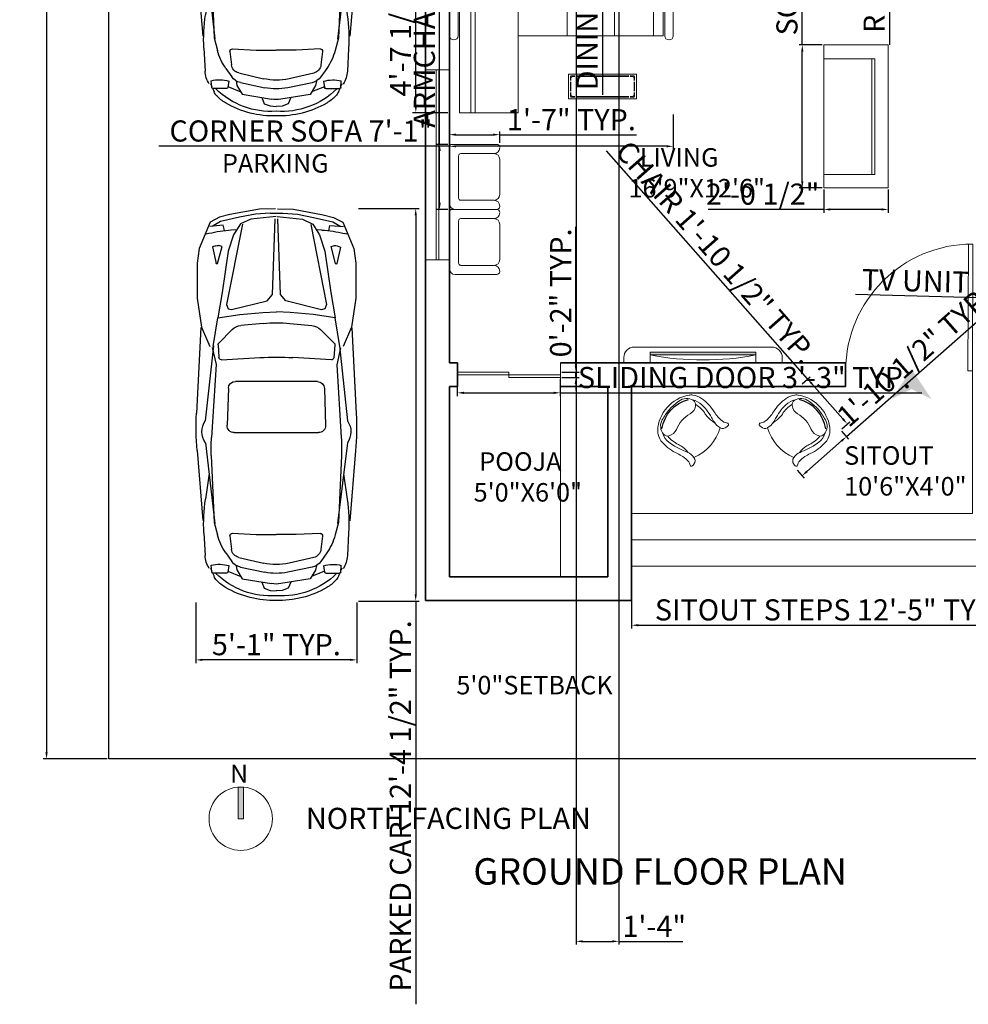
# Model space of a CAD drawing. Units: inches. Extents: x 3394 to 4794, y 965 to 1718.
# Tile 1 of 15: x 3394 to 3753, y 965 to 1338. Entities that reach past the tile are written whole.
import ezdxf

# ---------------------------------------------------------------- set-up
doc = ezdxf.new("R2010")
doc.units = ezdxf.units.IN
for name, color, linetype, lineweight in [('A-ANNO-DIMS', 2, 'Continuous', 13), ('A-ANNO-PATT', 1, 'Continuous', 13), ('A-ANNO-SYMB', 7, 'Continuous', 18), ('A-ANNO-TEXT', 7, 'Continuous', 18), ('A-ANNO-TITL', 7, 'Continuous', 25), ('A-AREA-IDEN', 7, 'Continuous', 18), ('A-DOOR', 4, 'Continuous', 18), ('A-EQPM', 8, 'Continuous', 18), ('A-EQPM-PATT', 8, 'Continuous', 13), ('A-FLOR-CASE', 8, 'Continuous', 18), ('A-FLOR-STRS', 7, 'Continuous', 18), ('A-GLAZ', 4, 'Continuous', 18), ('A-WALL', 7, 'Continuous', 35), ('C-PRKG-VEHI', 8, 'Continuous', 13), ('C-PROP', 7, 'Continuous', 25), ('NOITHAT', 21, 'Continuous', 18)]:
    doc.layers.add(name, color=color, linetype=linetype, lineweight=lineweight)
doc.layers.add('IFF-FURN-DETAIL', color=250, linetype='Continuous')
doc.layers.add('L9012X$0', color=2, linetype='Continuous')
doc.styles.get("Standard").update_dxf_attribs({"font": 'arial.ttf'})
doc.dimstyles.new('ISO-25', dxfattribs={"dimtxt": 8, "dimasz": 2.5, "dimexe": 1.25, "dimexo": 0.625, "dimtad": 1, "dimlunit": 3, "dimtxsty": 'Standard', "dimcen": 2.5, "dimadec": 0, "dimazin": 0, "dimtfac": 1, "dimtmove": 0, "dimatfit": 3, "dimfxl": 1, "dimarcsym": 0})

# ---------------------------------------------------------------- blocks, each defined once
blk = doc.blocks.new('sofa-27')
at = {"color": 0, "linetype": 'ByBlock'}
for p, q in [((0.094, 0.52), (0.459, 0.52)), ((-0.059, 0.059), (-0.059, 0.49)), ((0.035, 0.118), (0.035, 0.461)), ((0.518, 0.118), (0.518, 0.461)), ((0.613, 0.03), (0.613, 0.49)), ((0.583, 0), (0, 0)), ((0.494, 0.094), (0.059, 0.094))]:
    blk.add_line(p, q, dxfattribs=at)
for centre, radius, start, end in [((-0.03, 0.49), 0.0295, 90, 180), ((-0.024, 0.461), 0.0591, 360, 90), ((0.094, 0.461), 0.0591, 90, 180), ((0.459, 0.461), 0.0591, 0, 90), ((0.577, 0.461), 0.0591, 90, 180), ((0.583, 0.49), 0.0295, 0, 90), ((0.059, 0.118), 0.0236, 180, 270), ((0.494, 0.118), 0.0236, 270, 0), ((0, 0.059), 0.0591, 180, 270), ((0.583, 0.03), 0.0295, 270, 0)]:
    blk.add_arc(centre, radius, start, end, dxfattribs=at)
blk = doc.blocks.new('ILNG95')
for points in [[(120, 308, -0.32971), (51, 384, -0.036099), (50, 422, -0.497733), (75, 439, -0.070621), (96, 429, 0.101868), (133, 414, 0.091794), (259, 412, 0.024114), (351, 433, -0.090294), (638, 458, -0.132412), (775, 407, -0.068618), (816, 368, -0.184346), (943, 0, 1.803905)], [(120, 308, 0.138132), (244, 313, 0.001085), (325, 339, -0.034227), (462, 375, -0.033255), (567, 387, -0.137428), (727, 350, -4.561553)], [(120, 308, 0.138132), (244, 313, 0.001085), (325, 339, -0.034227), (462, 375, -0.033255), (567, 387, -0.137428), (727, 350, -4.561553)], [(235, 308, 0.064243), (394, 307, 0.04414), (433, 315, -0.118032), (643, 329, -6.296816)], [(235, 308, 0.064243), (394, 307, 0.04414), (433, 315, -0.118032), (643, 329, -6.296816)], [(639, 0, 0.078302), (612, 161, -0.233633), (633, 315, -0.28763), (710, 349, -0.317923), (875, 193, -0.032882), (900, 0, 1.140397)], [(639, 0, 0.078302), (612, 161, -0.233633), (633, 315, -0.28763), (710, 349, -0.317923), (875, 193, -0.032882), (900, 0, 1.140397)], [(120, -308, 0.32971), (51, -384, 0.036099), (50, -422, 0.497733), (75, -439, 0.070621), (96, -429, -0.101868), (133, -414, -0.091794), (259, -412, -0.024114), (351, -433, 0.090294), (638, -458, 0.132412), (775, -407, 0.068618), (816, -368, 0.184346), (943, 0, -1.803905)], [(639, 0, -0.078302), (612, -161, 0.233633), (633, -315, 0.28763), (710, -349, 0.317923), (875, -193, 0.032882), (900, 0, -1.140397)], [(639, 0, -0.078302), (612, -161, 0.233633), (633, -315, 0.28763), (710, -349, 0.317923), (875, -193, 0.032882), (900, 0, -1.140397)], [(120, -308, -0.138132), (244, -313, -0.001085), (325, -339, 0.034227), (462, -375, 0.033255), (567, -387, 0.137428), (727, -350, 4.561553)], [(120, -308, -0.138132), (244, -313, -0.001085), (325, -339, 0.034227), (462, -375, 0.033255), (567, -387, 0.137428), (727, -350, 4.561553)], [(235, -308, -0.064243), (394, -307, -0.04414), (433, -315, 0.118032), (643, -329, 6.296816)], [(235, -308, -0.064243), (394, -307, -0.04414), (433, -315, 0.118032), (643, -329, 6.296816)]]:
    blk.add_lwpolyline(points, format="xyb")
blk.add_arc((759, 1), 709, 154.3281, 205.801)
at = {"layer": 'IFF-FURN-DETAIL'}
blk.add_arc((326, -2), 549, 326.8997, 34.6691, dxfattribs=at)
blk.add_arc((326, -2), 549, 326.8997, 34.6691, dxfattribs=at)
blk = doc.blocks.new('A1099DC')
at = {"color": 0, "linetype": 'ByBlock'}
for p, q in [((1279.298465, 804.448389), (2201.430588, 851.890505)), ((272.228253, 749.073842), (265.114727, 718.465169)), ((1475.52921, 670.226262), (2282.402739, 758.004075)), ((2519.280414, 756.817792), (3387.476361, 653.818028)), ((2602.736326, 846.078152), (3356.693814, 785.353187)), ((2851.341839, 715.213377), (3126.60716, 755.701993)), ((3488.458929, 772.663345), (3732.658862, 759.86454)), ((139.051458, 595.027331), (190.951238, 683.213377)), ((179.200345, 564.515703), (190.951238, 709.631982)), ((398.733388, 644.315148), (411.280494, 678.748261)), ((411.280494, 678.748261), (588.616917, 641.417897)), ((1482.852352, 674.283145), (1175.286956, 622.180789)), ((1494.603245, 682.841284), (1678.210958, 641.166865)), ((1678.210958, 641.166865), (2462.684993, 690.847736)), ((2656.476214, 692.831247), (3376.704709, 662.004075)), ((3376.704709, 662.004075), (3510.708679, 626.736433)), ((3909.27561, 688.812956), (3837.725727, 693.401722)), ((3867.794139, 700.329656), (3900.059395, 686.767505)), ((3921.162781, 527.618662), (3921.162781, 676.138994)), ((3925.383812, 676.122818), (3955.306409, 663.545364)), ((92.537504, 388.14361), (139.051458, 595.027331)), ((236.043912, 551.980927), (179.200345, 564.515703)), ((405.405047, 577.538958), (396.874865, 615.894428)), ((589.014326, 626.599587), (405.405047, 577.538958)), ((1300.814287, 466.658131), (1445.712032, 613.104998)), ((1465.665584, 620.56924), (1602.893878, 610.287296)), ((1626.354615, 583.507504), (1602.652901, 169.222264)), ((3704.596898, 536.993674), (3795.675135, 473.385795)), ((229.117398, 477.634662), (225.714299, 427.957563)), ((1860.238743, -448.635916), (1859.369151, 433.397797)), ((1933.148906, 509.557888), (2330.980062, 522.200075)), ((2409.60024, 445.938054), (2410.49349, -460.09121)), ((3493.960271, 465.734554), (3507.923021, 209.166865)), ((3522.252709, 492.345257), (3666.066199, 475.644444)), ((3839.396146, 426.841284), (3888.358202, 417.538958)), ((3841.786866, 503.451367), (3910.58243, 515.096797)), ((3901.001848, 514.780764), (3957.150905, 375.772812)), ((57.774444, 216.608726), (92.537504, 388.14361)), ((1235.045743, 136.116317), (1257.419842, 373.755108)), ((3753.293176, 397.789551), (3815.226005, 132.124765)), ((3857.610793, 379.525702), (3912.067615, 118.157673)), ((3888.358202, 417.538958), (3983.199613, 359.957848)), ((3983.199613, 359.957848), (4035.448301, 43.94997)), ((49.168662, 58.00681), (57.774444, 216.608726)), ((3507.923021, 209.166865), (3507.64153, -4.333678)), ((4019.086894, 150.376168), (4084.69605, 122.469191)), ((4084.69605, 122.469191), (4109.177079, 60.329656)), ((4109.177079, 60.329656), (4113.094043, -5.158716)), ((49.301278, -76.507426), (58.219773, -235.092064)), ((3508.347273, -221.154823), (3507.644805, -7.65525)), ((3983.920268, -371.008369), (4035.545755, -54.898082)), ((4084.948231, -133.320044), (4109.306686, -71.132359)), ((4109.306686, -71.132359), (4113.094514, -5.636391)), ((1235.330373, -152.586046), (1258.173002, -390.180259)), ((1627.520644, -599.204785), (1603.002095, -184.967086)), ((3754.088875, -409.293325), (3815.497749, -143.506937)), ((3858.370276, -390.823819), (3912.311631, -129.348921)), ((4019.394229, -161.356334), (4084.948231, -133.320044)), ((58.219773, -235.092064), (93.320996, -406.558069)), ((3494.890446, -477.749545), (3508.347273, -221.154823)), ((93.320996, -406.558069), (140.24279, -613.349673)), ((3889.19258, -428.776374), (3983.920268, -371.008369)), ((3902.027941, -525.993061), (3957.902795, -386.874665)), ((230.077082, -495.779641), (226.576036, -446.109349)), ((1301.750547, -482.997536), (1446.936772, -629.158411)), ((1934.168526, -524.650381), (2332.023837, -536.508105)), ((3523.2353, -504.304409), (3667.01558, -487.320059)), ((3705.667171, -548.593196), (3796.61981, -484.805853)), ((3840.248961, -438.175225), (3889.19258, -428.776374)), ((3842.790735, -514.780444), (3911.609128, -526.290202)), ((140.24279, -613.349673), (192.316354, -701.433212)), ((237.150178, -570.112104), (180.331436, -582.758939)), ((180.331436, -582.758939), (192.368445, -727.851766)), ((406.561378, -595.336142), (398.106841, -633.708356)), ((590.267037, -644.034637), (406.561378, -595.336142)), ((1466.905004, -636.583294), (1604.112757, -626.030785)), ((3922.214148, -538.79118), (3922.506998, -687.311224)), ((273.723073, -767.133288), (266.549207, -736.538701)), ((400.0214, -662.125356), (412.636377, -696.533662)), ((412.636377, -696.533662), (589.898847, -658.853701)), ((1484.19765, -690.263206), (1176.530118, -638.767405)), ((1476.866524, -686.22077), (2283.911563, -772.40743)), ((1495.965396, -698.798158), (1679.490579, -656.761786)), ((1679.490579, -656.761786), (2464.061049, -704.895745)), ((2520.786439, -770.754078), (3388.777604, -666.042617)), ((2657.855804, -706.497136), (3378.022114, -674.249887)), ((2852.765183, -728.494989), (3128.109803, -768.440762)), ((3378.022114, -674.249887), (3511.956283, -638.718087)), ((3910.644841, -700.0086), (3839.104145, -704.738438)), ((3869.186159, -711.60707), (3901.424611, -697.981326)), ((3926.727989, -687.286725), (3956.625729, -674.650294)), ((1280.900818, -820.829563), (2203.124693, -866.453338)), ((2604.418191, -859.849707), (3358.254477, -797.638217)), ((3489.994314, -784.688586), (3734.168535, -771.408296))]:
    blk.add_line(p, q, dxfattribs=at)
for points in [[(-0.000783, 0.794772), (5.385043, 172.701749), (63.649891, 493.818028), (92.537504, 603.957563), (144.437284, 705.166865), (428.417214, 824.236633), (585.095796, 846.190121), (961.406447, 846.190121), (1274.27399, 797.818028), (1482.852352, 709.631982)], [(83.345007, -3.206171), (111.32237, 268.957533), (164.563706, 379.583828), (279.999271, 453.709838), (456.549665, 511.628518), (901.254996, 574.918954), (1175.286956, 622.180789), (1137.52997, 385.548359), (1118.345181, 137.317882), (1109.829198, -8.358455)], [(168.178729, 359.003083), (1030.214866, 528.397865), (1077.798844, 510.531569), (1086.170082, 475.285426), (992.832238, 91.960378), (924.218938, 35.478085), (108.447994, 6.034416)], [(0.019119, -19.392451), (5.743899, -191.288474), (64.641806, -512.289243), (93.746535, -622.371603), (145.845778, -723.478374), (430.059935, -841.987962), (586.7815, -863.632471), (963.091723, -863.198028), (1275.863278, -814.209121), (1484.26735, -725.611974)], [(83.356858, -15.227176), (111.870816, -287.335185), (165.330179, -397.856284), (280.911681, -471.754535), (457.575935, -529.324983), (902.4055, -592.045995), (1176.530118, -638.767405), (1138.306616, -402.209884), (1118.632407, -154.017717), (1109.829198, -8.358455)], [(168.904615, -377.268451), (1031.273389, -545.270714), (1078.822046, -527.310627), (1087.123771, -492.048047), (993.030273, -108.907787), (924.305735, -52.560894), (108.478017, -24.418246)]]:
    blk.add_lwpolyline(points, dxfattribs=at)
for centre, radius, start, end in [((2358.037832, -2192.08357), 3048, 85.395244, 92.945173), ((2399.99649, 588.663508), 206.166238, 54.649181, 124.776949), ((3392.740754, -1053.630025), 1828.8, 86.999806, 98.367602), ((3718.678317, 475.802507), 284.405862, 57.329946, 87.182375), ((1749.553982, 373.478072), 1524, 166.916578, 176.08111), ((446.46332, 626.922805), 50.8, 159.97873, 192.538409), ((587.047263, 633.961317), 7.62, 284.960009, 78.112462), ((2578.271641, -1134.295865), 1828.8, 87.549126, 93.623712), ((4191.049821, 605.937201), 363.988953, 166.096081, 196.353514), ((3908.462781, 676.138994), 12.7, 0, 86.330429), ((3320.85101, 50.338397), 847.430844, 356.245089, 44.519453), ((3896.252417, 523.051998), 152.4, 46.38363, 67.20138), ((1463.767788, 595.240237), 25.4, 85.715073, 135.304647), ((1600.996082, 584.958293), 25.4, 356.725615, 85.715073), ((3355.555414, 37.211519), 609.6, 55.070043, 75.255062), ((3700.933354, 318.064082), 435.542335, 30.457681, 46.38363), ((3204.184594, 25.950693), 1011.814461, 358.069446, 30.457681), ((1409.148822, 359.469565), 152.4, 135.304647, 174.62136), ((1935.569151, 433.396333), 76.2, 91.82012, 179.9989), ((2333.400307, 446.03852), 76.2, 359.924458, 91.82012), ((3519.322741, 467.114813), 25.4, 83.37601, 183.115039), ((3654.346327, 374.722669), 101.6, 13.122645, 83.37601), ((3708.414764, 348.440256), 152.4, 11.769371, 55.070043), ((3908.462781, 527.618662), 12.7, 279.607718, 0), ((2752.335538, -6.739118), 1524, 174.62136, 185.491615), ((4645.676894, -4.872483), 3048, 176.725615, 183.38736), ((3221.54491, -6.276527), 609.6, 346.99033, 13.122645), ((3315.283499, -6.18411), 609.6, 348.343604, 11.769371), ((1266.577845, -8.050136), 1219.2, 176.894161, 183.218814), ((3734.73098, -5.770579), 304.8, 350.724636, 9.388339), ((3320.962449, -62.69553), 847.430844, 315.593523, 3.867886), ((3204.248172, -38.537915), 1011.814461, 329.655294, 2.043529), ((1409.873518, -375.595566), 152.4, 185.491615, 224.808328), ((3655.096735, -386.42159), 101.6, 276.736965, 346.99033), ((3709.113243, -360.032616), 152.4, 305.042932, 348.343604), ((1750.305335, -388.625277), 1524, 184.031865, 193.196397), ((1936.438592, -448.484202), 76.2, 180.114076, 268.292856), ((2334.293902, -460.341926), 76.2, 268.292856, 0.188517), ((3520.255588, -479.079792), 25.4, 176.997936, 276.736965), ((4192.255091, -616.577407), 363.988953, 163.759461, 194.016894), ((3909.514173, -538.816222), 12.7, 0.112975, 80.505257), ((447.716945, -644.638934), 50.8, 167.574566, 200.134245), ((1464.957267, -611.258083), 25.4, 224.808328, 274.397903), ((1602.165021, -600.705574), 25.4, 274.397903, 3.38736), ((3355.640902, -49.500248), 609.6, 284.857913, 305.042932), ((3701.571953, -329.671253), 435.542335, 313.729345, 329.655294), ((588.314493, -651.400231), 7.62, 282.000513, 75.152966), ((2576.048678, 1120.472221), 1828.8, 266.489263, 272.563849), ((3719.627907, -487.374382), 284.405862, 272.930601, 302.78303), ((3909.807023, -687.336265), 12.7, 273.782546, 0.112975), ((3897.294828, -534.273643), 152.4, 292.911596, 313.729345), ((2401.171182, -602.835323), 206.166238, 235.336026, 305.463794), ((3390.675263, 1041.412497), 1828.8, 261.745373, 273.113169), ((2353.729565, 2177.823616), 3048, 267.167802, 274.717731)]:
    blk.add_arc(centre, radius, start, end, dxfattribs=at)
blk = doc.blocks.new('VI')
at = {"layer": 'L9012X$0'}
blk.add_blockref('A1099DC', (0, 0), dxfattribs=at)
blk = doc.blocks.new('TABLE-30A')
at = {"color": 0, "linetype": 'ByBlock'}
for p, q in [((0, 0), (0, 0.55)), ((0, 0.55), (1.5, 0.55)), ((0.051, 0.508), (0.042, 0.499)), ((0.042, 0.499), (0.042, 0.478)), ((0.042, 0.478), (0.072, 0.478)), ((0.042, 0.478), (0.042, 0.41)), ((0.072, 0.508), (0.051, 0.508)), ((0.051, 0.478), (0.051, 0.41)), ((0.072, 0.478), (0.072, 0.508)), ((0.072, 0.508), (0.14, 0.508)), ((0.072, 0.499), (0.14, 0.499)), ((1.331, 0.508), (0.169, 0.508)), ((1.331, 0.499), (0.169, 0.499)), ((1.428, 0.508), (1.36, 0.508)), ((1.428, 0.499), (1.36, 0.499)), ((1.428, 0.508), (1.428, 0.478)), ((1.449, 0.508), (1.428, 0.508)), ((1.428, 0.478), (1.458, 0.478)), ((1.458, 0.499), (1.449, 0.508)), ((1.449, 0.478), (1.449, 0.41)), ((1.458, 0.478), (1.458, 0.499)), ((1.458, 0.478), (1.458, 0.41)), ((1.5, 0.55), (1.5, 0)), ((0.042, 0.169), (0.042, 0.381)), ((0.051, 0.169), (0.051, 0.381)), ((1.449, 0.381), (1.449, 0.169)), ((1.458, 0.381), (1.458, 0.169)), ((1.5, 0), (0, 0)), ((0.042, 0.072), (0.042, 0.14)), ((0.042, 0.072), (0.042, 0.051)), ((0.072, 0.072), (0.042, 0.072)), ((0.042, 0.051), (0.051, 0.042)), ((0.051, 0.072), (0.051, 0.14)), ((0.051, 0.042), (0.072, 0.042)), ((0.072, 0.042), (0.072, 0.072)), ((0.072, 0.051), (0.14, 0.051)), ((0.072, 0.042), (0.14, 0.042)), ((0.169, 0.051), (1.331, 0.051)), ((0.169, 0.042), (1.331, 0.042)), ((1.428, 0.051), (1.36, 0.051)), ((1.428, 0.042), (1.36, 0.042)), ((1.428, 0.072), (1.428, 0.042)), ((1.458, 0.072), (1.428, 0.072)), ((1.428, 0.042), (1.449, 0.042)), ((1.449, 0.072), (1.449, 0.14)), ((1.449, 0.042), (1.458, 0.051)), ((1.458, 0.072), (1.458, 0.14)), ((1.458, 0.051), (1.458, 0.072))]:
    blk.add_line(p, q, dxfattribs=at)
blk = doc.blocks.new('12')
at = {"color": 0}
for p, q in [((5656.26, 3021.25), (5553.9, 3021.25)), ((5553.9, 3021.25), (5553.9, 2989.76)), ((5557.83, 3021.25), (5557.83, 2989.76)), ((5656.26, 2989.76), (5656.26, 3021.25)), ((5652.32, 3017.31), (5558.49, 3017.31)), ((5558.49, 3017.31), (5558.49, 2989.76)), ((5562.89, 3017.31), (5562.89, 2989.76)), ((5580.8, 3017.31), (5580.8, 2989.76)), ((5602.45, 3017.31), (5602.45, 2989.76)), ((5624.76, 3017.31), (5624.76, 2954.53)), ((5651.66, 3017.31), (5651.66, 2954.53)), ((5652.32, 2989.76), (5652.32, 3017.31)), ((5646.42, 3011.41), (5558.49, 3011.41)), ((5644.45, 3009.44), (5558.49, 3009.44)), ((5644.45, 2954.53), (5644.45, 3009.44)), ((5646.42, 2954.53), (5646.42, 3011.41)), ((5624.76, 2995), (5624.76, 2954.53)), ((5558.49, 2989.76), (5624.76, 2989.76)), ((5651.66, 2954.53), (5624.76, 2954.53))]:
    blk.add_line(p, q, dxfattribs=at)
for centre in [(5555.86, 2989.76), (5654.29, 2989.76)]:
    blk.add_arc(centre, 1.97, 180, 0, dxfattribs=at)
at = {"xscale": -20.70834898381633, "yscale": 20.70834898381633, "zscale": 20.70834898381633}
blk.add_blockref('TABLE-30A', (5601.8, 2960.82), dxfattribs=at)
blk = doc.blocks.new('12PCOU24')
for p, q in [((9.63, 33.87), (9.63, -34.12)), ((38, 33.87), (38, -34.12))]:
    blk.add_line(p, q)
blk.add_lwpolyline([(0, 42.12), (38, 42.12), (38, 33.87), (8, 33.87), (8, -34.12), (38, -34.12), (38, -42.12), (0, -42.12)], close=True)
blk = doc.blocks.new('*D31')
at = {"layer": 'A-ANNO-DIMS', "color": 0, "lineweight": -2, "transparency": 16777216}
for p, q in [((3427.12, 1666.68), (3402.95, 1666.68)), ((3404.2, 1664.18), (3404.2, 1060.18)), ((3427.12, 1057.68), (3402.95, 1057.68))]:
    blk.add_line(p, q, dxfattribs=at)
at = {"layer": 'A-ANNO-DIMS', "color": 0, "transparency": 16777216}
for points in [[(3403.78, 1664.18), (3404.62, 1664.18), (3404.2, 1666.68)], [(3403.78, 1060.18), (3404.62, 1060.18), (3404.2, 1057.68)]]:
    blk.add_solid(points, dxfattribs=at)
at = {"layer": 'Defpoints', "color": 0, "transparency": 16777216}
for p in [(3427.74, 1666.68), (3404.2, 1057.68), (3427.74, 1057.68)]:
    blk.add_point(p, dxfattribs=at)
at = {"layer": 'A-ANNO-DIMS', "color": 0, "transparency": 16777216, "insert": (3399.49, 1362.18), "char_height": 8, "attachment_point": 5, "rotation": 90}
blk.add_mtext('50\'-9"', dxfattribs=at)
blk = doc.blocks.new('WIN-72IN')
for p, q in [((9, 72), (0, 72)), ((4, 0), (4, 72)), ((5, 0), (5, 72)), ((9, 0), (0, 0))]:
    blk.add_line(p, q)
blk = doc.blocks.new('DOOR-ENTRY-48IN')
for p, q in [((0.03, 6.2), (0, 0.2)), ((48.03, 6), (48, 0))]:
    blk.add_line(p, q)
blk.add_lwpolyline([(48.03, 6), (48.24, 54), (46.49, 54.01), (46.28, 6.01)], close=True)
blk.add_arc((48.03, 6), 48, 90, 179.759)
blk = doc.blocks.new('DOOR-SLIDING-39IN')
for p, q in [((0, 2), (19.5, 2)), ((0, 1), (39, 1)), ((19.5, 2), (19.5, 0)), ((19.5, 0), (39, 0))]:
    blk.add_line(p, q)
blk = doc.blocks.new('NORTH-ARROW-PLAN')
at = {"transparency": 33554687}
h = blk.add_hatch(color=256, dxfattribs=at)
h.dxf.hatch_style = 1
h.paths.add_polyline_path([(13, 12), (11, 12), (11, 23.96, -0.020861), (12, 24, -0.020861), (13, 23.96)])
for p, q in [((11, 24), (11, 12)), ((13, 12), (13, 23.96)), ((11, 12), (13, 12))]:
    blk.add_line(p, q)
blk.add_circle((12, 12), 12)
blk.add_text('N', height=6.9).set_placement((7.98, 25.6))
blk = doc.blocks.new('STAIR-SITOUT-3STEP')
for p, q in [((129, 68), (129, 20)), ((139, 68), (139, 10)), ((149, 68), (149, 0)), ((0, 20), (129, 20)), ((0, 10), (139, 10)), ((0, 0), (149, 0))]:
    blk.add_line(p, q)
blk = doc.blocks.new('*D70')
at = {"layer": 'A-ANNO-DIMS', "color": 0, "lineweight": -2, "transparency": 16777216}
for p, q in [((3559.74, 1201.56), (3559.74, 1195.08)), ((3598.74, 1201.56), (3598.74, 1195.08)), ((3562.24, 1196.33), (3596.24, 1196.33)), ((3598.74, 1196.33), (3735.67, 1196.33))]:
    blk.add_line(p, q, dxfattribs=at)
at = {"layer": 'A-ANNO-DIMS', "color": 0, "transparency": 16777216}
for points in [[(3562.24, 1196.75), (3562.24, 1195.92), (3559.74, 1196.33)], [(3596.24, 1196.75), (3596.24, 1195.92), (3598.74, 1196.33)]]:
    blk.add_solid(points, dxfattribs=at)
at = {"layer": 'Defpoints', "color": 0, "transparency": 16777216}
for p in [(3559.74, 1202.18), (3598.74, 1202.18), (3598.74, 1196.33)]:
    blk.add_point(p, dxfattribs=at)
at = {"layer": 'A-ANNO-DIMS', "color": 0, "transparency": 16777216, "insert": (3668.46, 1201.1), "char_height": 8, "attachment_point": 5}
blk.add_mtext('SLIDING DOOR 3\'-3" TYP.', dxfattribs=at)
blk = doc.blocks.new('*D71')
at = {"layer": 'A-ANNO-DIMS', "color": 0, "lineweight": -2, "transparency": 16777216}
for p, q in [((3604.59, 1206.68), (3604.59, 1259.2)), ((3599.37, 1204.18), (3605.84, 1204.18)), ((3599.37, 1202.18), (3605.84, 1202.18)), ((3604.59, 1202.18), (3604.59, 1204.18)), ((3604.59, 1199.68), (3604.59, 1197.18))]:
    blk.add_line(p, q, dxfattribs=at)
at = {"layer": 'A-ANNO-DIMS', "color": 0, "transparency": 16777216}
for points in [[(3604.18, 1206.68), (3605.01, 1206.68), (3604.59, 1204.18)], [(3604.18, 1199.68), (3605.01, 1199.68), (3604.59, 1202.18)]]:
    blk.add_solid(points, dxfattribs=at)
at = {"layer": 'Defpoints', "color": 0, "transparency": 16777216}
for p in [(3598.74, 1204.18), (3598.74, 1202.18), (3604.59, 1204.18)]:
    blk.add_point(p, dxfattribs=at)
at = {"layer": 'A-ANNO-DIMS', "color": 0, "transparency": 16777216, "insert": (3599.89, 1234.19), "char_height": 8, "attachment_point": 5, "rotation": 90}
blk.add_mtext('0\'-2" TYP.', dxfattribs=at)
blk = doc.blocks.new('*D72')
at = {"layer": 'A-ANNO-DIMS', "color": 0, "lineweight": -2, "transparency": 16777216}
for p, q in [((3625.74, 1130.06), (3625.74, 1107.08)), ((3774.74, 1130.06), (3774.74, 1107.08)), ((3628.24, 1108.33), (3772.24, 1108.33))]:
    blk.add_line(p, q, dxfattribs=at)
at = {"layer": 'A-ANNO-DIMS', "color": 0, "transparency": 16777216}
for points in [[(3628.24, 1108.75), (3628.24, 1107.92), (3625.74, 1108.33)], [(3772.24, 1108.75), (3772.24, 1107.92), (3774.74, 1108.33)]]:
    blk.add_solid(points, dxfattribs=at)
at = {"layer": 'Defpoints', "color": 0, "transparency": 16777216}
for p in [(3625.74, 1130.68), (3774.74, 1130.68), (3774.74, 1108.33)]:
    blk.add_point(p, dxfattribs=at)
at = {"layer": 'A-ANNO-DIMS', "color": 0, "transparency": 16777216, "insert": (3700.24, 1113.1), "char_height": 8, "attachment_point": 5}
blk.add_mtext('SITOUT STEPS 12\'-5" TYP.', dxfattribs=at)
blk = doc.blocks.new('*D74')
at = {"layer": 'A-ANNO-DIMS', "color": 0, "lineweight": -2, "transparency": 16777216}
for p, q in [((3522.32, 1266.09), (3545.23, 1266.09)), ((3543.98, 1263.59), (3543.98, 1120)), ((3522.32, 1117.5), (3545.23, 1117.5)), ((3543.98, 1117.5), (3543.98, 964.77))]:
    blk.add_line(p, q, dxfattribs=at)
at = {"layer": 'A-ANNO-DIMS', "color": 0, "transparency": 16777216}
for points in [[(3543.57, 1263.59), (3544.4, 1263.59), (3543.98, 1266.09)], [(3543.57, 1120), (3544.4, 1120), (3543.98, 1117.5)]]:
    blk.add_solid(points, dxfattribs=at)
at = {"layer": 'Defpoints', "color": 0, "transparency": 16777216}
for p in [(3521.7, 1266.09), (3521.7, 1117.5), (3543.98, 1117.5)]:
    blk.add_point(p, dxfattribs=at)
at = {"layer": 'A-ANNO-DIMS', "color": 0, "transparency": 16777216, "insert": (3539.22, 1039.89), "char_height": 8, "attachment_point": 5, "rotation": 90}
blk.add_mtext('PARKED CAR 12\'-4 1/2" TYP.', dxfattribs=at)
blk = doc.blocks.new('*D75')
at = {"layer": 'A-ANNO-DIMS', "color": 0, "lineweight": -2, "transparency": 16777216}
for p, q in [((3460.75, 1116.88), (3460.75, 1093.97)), ((3521.7, 1116.88), (3521.7, 1093.97)), ((3519.2, 1095.22), (3463.25, 1095.22))]:
    blk.add_line(p, q, dxfattribs=at)
at = {"layer": 'A-ANNO-DIMS', "color": 0, "transparency": 16777216}
for points in [[(3463.25, 1095.63), (3463.25, 1094.8), (3460.75, 1095.22)], [(3519.2, 1095.63), (3519.2, 1094.8), (3521.7, 1095.22)]]:
    blk.add_solid(points, dxfattribs=at)
at = {"layer": 'Defpoints', "color": 0, "transparency": 16777216}
for p in [(3460.75, 1117.5), (3521.7, 1117.5), (3460.75, 1095.22)]:
    blk.add_point(p, dxfattribs=at)
at = {"layer": 'A-ANNO-DIMS', "color": 0, "transparency": 16777216, "insert": (3491.22, 1099.93), "char_height": 8, "attachment_point": 5}
blk.add_mtext('5\'-1" TYP.', dxfattribs=at)
blk = doc.blocks.new('*D76')
at = {"layer": 'A-ANNO-DIMS', "color": 0, "lineweight": -2, "transparency": 16777216}
for p, q in [((3553.05, 1290.42), (3553.05, 1424.75)), ((3556.12, 1290.42), (3551.8, 1290.42)), ((3553.05, 1268.3), (3553.05, 1287.92)), ((3556.12, 1265.8), (3551.8, 1265.8))]:
    blk.add_line(p, q, dxfattribs=at)
at = {"layer": 'A-ANNO-DIMS', "color": 0, "transparency": 16777216}
for points in [[(3552.63, 1287.92), (3553.47, 1287.92), (3553.05, 1290.42)], [(3552.63, 1268.3), (3553.47, 1268.3), (3553.05, 1265.8)]]:
    blk.add_solid(points, dxfattribs=at)
at = {"layer": 'Defpoints', "color": 0, "transparency": 16777216}
for p in [(3553.05, 1290.42), (3556.74, 1290.42), (3556.74, 1265.8)]:
    blk.add_point(p, dxfattribs=at)
at = {"layer": 'A-ANNO-DIMS', "color": 0, "transparency": 16777216, "insert": (3548.29, 1358.84), "char_height": 8, "attachment_point": 5, "rotation": 90}
blk.add_mtext('ARMCHAIR 2\'-0 1/2" TYP.', dxfattribs=at)
blk = doc.blocks.new('*D77')
at = {"layer": 'A-ANNO-DIMS', "color": 0, "lineweight": -2, "transparency": 16777216}
for p, q in [((3556.74, 1291.04), (3556.74, 1295.36)), ((3559.24, 1294.11), (3573.3, 1294.11)), ((3575.8, 1291.04), (3575.8, 1295.36)), ((3575.8, 1294.11), (3627.56, 1294.11))]:
    blk.add_line(p, q, dxfattribs=at)
at = {"layer": 'A-ANNO-DIMS', "color": 0, "transparency": 16777216}
for points in [[(3559.24, 1294.53), (3559.24, 1293.7), (3556.74, 1294.11)], [(3573.3, 1294.53), (3573.3, 1293.7), (3575.8, 1294.11)]]:
    blk.add_solid(points, dxfattribs=at)
at = {"layer": 'Defpoints', "color": 0, "transparency": 16777216}
for p in [(3575.8, 1294.11), (3556.74, 1290.42), (3575.8, 1290.42)]:
    blk.add_point(p, dxfattribs=at)
at = {"layer": 'A-ANNO-DIMS', "color": 0, "transparency": 16777216, "insert": (3602.93, 1298.76), "char_height": 8, "attachment_point": 5}
blk.add_mtext('1\'-7" TYP.', dxfattribs=at)
blk = doc.blocks.new('*D82')
at = {"layer": 'A-ANNO-DIMS', "color": 0, "lineweight": -2, "transparency": 16777216}
for p, q in [((3692.34, 1201.63), (3616.17, 1287.99)), ((3690.25, 1199.79), (3693.28, 1202.46)), ((3705.73, 1186.44), (3693.99, 1199.75)), ((3705.29, 1182.73), (3708.32, 1185.4))]:
    blk.add_line(p, q, dxfattribs=at)
at = {"layer": 'A-ANNO-DIMS', "color": 0, "transparency": 16777216}
for points in [[(3694.3, 1200.03), (3693.68, 1199.48), (3692.34, 1201.63)], [(3706.04, 1186.72), (3705.42, 1186.17), (3707.38, 1184.57)]]:
    blk.add_solid(points, dxfattribs=at)
at = {"layer": 'Defpoints', "color": 0, "transparency": 16777216}
for p in [(3692.34, 1201.63), (3689.78, 1199.37), (3704.83, 1182.31)]:
    blk.add_point(p, dxfattribs=at)
at = {"layer": 'A-ANNO-DIMS', "color": 0, "transparency": 16777216, "insert": (3657, 1248.9), "char_height": 8, "attachment_point": 5, "rotation": 311.4119}
blk.add_mtext('CHAIR 1\'-10 1/2" TYP.', dxfattribs=at)
blk = doc.blocks.new('*D83')
at = {"layer": 'A-ANNO-DIMS', "color": 0, "lineweight": -2, "transparency": 16777216}
for p, q in [((3707.08, 1179.75), (3764.54, 1230.43)), ((3705.24, 1181.84), (3707.91, 1178.82)), ((3692.13, 1166.56), (3705.21, 1178.1)), ((3688.41, 1167), (3691.08, 1163.97))]:
    blk.add_line(p, q, dxfattribs=at)
at = {"layer": 'A-ANNO-DIMS', "color": 0, "transparency": 16777216}
for points in [[(3704.93, 1178.41), (3705.48, 1177.79), (3707.08, 1179.75)], [(3691.85, 1166.87), (3692.4, 1166.25), (3690.25, 1164.91)]]:
    blk.add_solid(points, dxfattribs=at)
at = {"layer": 'Defpoints', "color": 0, "transparency": 16777216}
for p in [(3704.83, 1182.31), (3707.08, 1179.75), (3687.99, 1167.47)]:
    blk.add_point(p, dxfattribs=at)
at = {"layer": 'A-ANNO-DIMS', "color": 0, "transparency": 16777216, "insert": (3733.6, 1209.49), "char_height": 8, "attachment_point": 5, "rotation": 41.4119}
blk.add_mtext('1\'-10 1/2" TYP.', dxfattribs=at)
blk = doc.blocks.new('*D84')
at = {"layer": 'A-ANNO-DIMS', "color": 0, "lineweight": -2, "transparency": 16777216}
for p, q in [((3828.32, 1230.52), (3710.44, 1233.52)), ((3828.15, 1223.75), (3828.35, 1231.77)), ((3875.11, 1229.33), (3830.82, 1230.46)), ((3877.44, 1222.5), (3877.64, 1230.51))]:
    blk.add_line(p, q, dxfattribs=at)
at = {"layer": 'A-ANNO-DIMS', "color": 0, "transparency": 16777216}
for points in [[(3830.83, 1230.87), (3830.81, 1230.04), (3828.32, 1230.52)], [(3875.12, 1229.75), (3875.1, 1228.91), (3877.61, 1229.27)]]:
    blk.add_solid(points, dxfattribs=at)
at = {"layer": 'Defpoints', "color": 0, "transparency": 16777216}
for p in [(3828.32, 1230.52), (3828.13, 1223.13), (3877.42, 1221.87)]:
    blk.add_point(p, dxfattribs=at)
at = {"layer": 'A-ANNO-DIMS', "color": 0, "transparency": 16777216, "insert": (3768.25, 1236.81), "char_height": 8, "attachment_point": 5, "rotation": 358.5431}
blk.add_mtext('TV UNIT 4\'-1 1/2" TYP.', dxfattribs=at)
blk = doc.blocks.new('*D90')
at = {"layer": 'A-ANNO-DIMS', "color": 0, "lineweight": -2, "transparency": 16777216}
for p, q in [((3728.12, 1480.68), (3722.09, 1480.68)), ((3723.34, 1478.18), (3723.34, 1447.18)), ((3728.12, 1444.68), (3722.09, 1444.68)), ((3723.34, 1444.68), (3723.34, 1328.18))]:
    blk.add_line(p, q, dxfattribs=at)
at = {"layer": 'A-ANNO-DIMS', "color": 0, "transparency": 16777216}
for points in [[(3722.93, 1478.18), (3723.76, 1478.18), (3723.34, 1480.68)], [(3722.93, 1447.18), (3723.76, 1447.18), (3723.34, 1444.68)]]:
    blk.add_solid(points, dxfattribs=at)
at = {"layer": 'Defpoints', "color": 0, "transparency": 16777216}
for p in [(3728.74, 1480.68), (3723.34, 1444.68), (3728.74, 1444.68)]:
    blk.add_point(p, dxfattribs=at)
at = {"layer": 'A-ANNO-DIMS', "color": 0, "transparency": 16777216, "insert": (3718.58, 1385.18), "char_height": 8, "attachment_point": 5, "rotation": 90}
blk.add_mtext('REFRIGERATOR 3\'-0"', dxfattribs=at)
blk = doc.blocks.new('*D100')
at = {"layer": 'A-ANNO-DIMS', "color": 0, "lineweight": -2, "transparency": 16777216}
for p, q in [((3556.74, 1301.79), (3556.74, 1288.45)), ((3641.52, 1301.79), (3641.52, 1288.45)), ((3556.74, 1289.7), (3446.75, 1289.7)), ((3639.02, 1289.7), (3559.24, 1289.7))]:
    blk.add_line(p, q, dxfattribs=at)
at = {"layer": 'A-ANNO-DIMS', "color": 0, "transparency": 16777216}
for points in [[(3559.24, 1290.12), (3559.24, 1289.29), (3556.74, 1289.7)], [(3639.02, 1290.12), (3639.02, 1289.29), (3641.52, 1289.7)]]:
    blk.add_solid(points, dxfattribs=at)
at = {"layer": 'Defpoints', "color": 0, "transparency": 16777216}
for p in [(3556.74, 1302.42), (3641.52, 1302.42), (3556.74, 1289.7)]:
    blk.add_point(p, dxfattribs=at)
at = {"layer": 'A-ANNO-DIMS', "color": 0, "transparency": 16777216, "insert": (3500.5, 1294.47), "char_height": 8, "attachment_point": 5}
blk.add_mtext('CORNER SOFA 7\'-1"', dxfattribs=at)
blk = doc.blocks.new('*D101')
at = {"layer": 'A-ANNO-DIMS', "color": 0, "lineweight": -2, "transparency": 16777216}
for p, q in [((3556.12, 1357.68), (3542.78, 1357.68)), ((3544.03, 1304.92), (3544.03, 1355.18)), ((3556.12, 1302.42), (3542.78, 1302.42))]:
    blk.add_line(p, q, dxfattribs=at)
at = {"layer": 'A-ANNO-DIMS', "color": 0, "transparency": 16777216}
for points in [[(3543.61, 1355.18), (3544.44, 1355.18), (3544.03, 1357.68)], [(3543.61, 1304.92), (3544.44, 1304.92), (3544.03, 1302.42)]]:
    blk.add_solid(points, dxfattribs=at)
at = {"layer": 'Defpoints', "color": 0, "transparency": 16777216}
for p in [(3544.03, 1357.68), (3556.74, 1357.68), (3556.74, 1302.42)]:
    blk.add_point(p, dxfattribs=at)
at = {"layer": 'A-ANNO-DIMS', "color": 0, "transparency": 16777216, "insert": (3539.27, 1330.05), "char_height": 8, "attachment_point": 5, "rotation": 90}
blk.add_mtext('4\'-7 1/2"', dxfattribs=at)
blk = doc.blocks.new('*D102')
at = {"layer": 'A-ANNO-DIMS', "color": 0, "lineweight": -2, "transparency": 16777216}
for p, q in [((3690.36, 1328.09), (3690.36, 1386.6)), ((3697.86, 1328.09), (3689.11, 1328.09)), ((3690.36, 1276.43), (3690.36, 1325.59)), ((3697.86, 1273.93), (3689.11, 1273.93))]:
    blk.add_line(p, q, dxfattribs=at)
at = {"layer": 'A-ANNO-DIMS', "color": 0, "transparency": 16777216}
for points in [[(3689.94, 1325.59), (3690.77, 1325.59), (3690.36, 1328.09)], [(3689.94, 1276.43), (3690.77, 1276.43), (3690.36, 1273.93)]]:
    blk.add_solid(points, dxfattribs=at)
at = {"layer": 'Defpoints', "color": 0, "transparency": 16777216}
for p in [(3690.36, 1328.09), (3698.48, 1328.09), (3698.48, 1273.93)]:
    blk.add_point(p, dxfattribs=at)
at = {"layer": 'A-ANNO-DIMS', "color": 0, "transparency": 16777216, "insert": (3685.59, 1358.6), "char_height": 8, "attachment_point": 5, "rotation": 90}
blk.add_mtext('SOFA 4\'-6"', dxfattribs=at)
blk = doc.blocks.new('*D103')
at = {"layer": 'A-ANNO-DIMS', "color": 0, "lineweight": -2, "transparency": 16777216}
for p, q in [((3698.48, 1273.3), (3698.48, 1264.55)), ((3722.91, 1273.3), (3722.91, 1264.55)), ((3698.48, 1265.8), (3654.69, 1265.8)), ((3720.41, 1265.8), (3700.98, 1265.8))]:
    blk.add_line(p, q, dxfattribs=at)
at = {"layer": 'A-ANNO-DIMS', "color": 0, "transparency": 16777216}
for points in [[(3700.98, 1266.22), (3700.98, 1265.38), (3698.48, 1265.8)], [(3720.41, 1266.22), (3720.41, 1265.38), (3722.91, 1265.8)]]:
    blk.add_solid(points, dxfattribs=at)
at = {"layer": 'Defpoints', "color": 0, "transparency": 16777216}
for p in [(3698.48, 1273.93), (3722.91, 1273.93), (3698.48, 1265.8)]:
    blk.add_point(p, dxfattribs=at)
at = {"layer": 'A-ANNO-DIMS', "color": 0, "transparency": 16777216, "insert": (3675.34, 1270.56), "char_height": 8, "attachment_point": 5}
blk.add_mtext('2\'-0 1/2"', dxfattribs=at)
blk = doc.blocks.new('*D104')
at = {"layer": 'A-ANNO-DIMS', "color": 0, "lineweight": -2, "transparency": 16777216}
for p, q in [((3622.3, 1455.61), (3613.46, 1455.61)), ((3614.71, 1453.11), (3614.71, 1403.36)), ((3622.3, 1400.86), (3613.46, 1400.86)), ((3614.71, 1400.86), (3614.71, 1309.18))]:
    blk.add_line(p, q, dxfattribs=at)
at = {"layer": 'A-ANNO-DIMS', "color": 0, "transparency": 16777216}
for points in [[(3614.29, 1453.11), (3615.13, 1453.11), (3614.71, 1455.61)], [(3614.29, 1403.36), (3615.13, 1403.36), (3614.71, 1400.86)]]:
    blk.add_solid(points, dxfattribs=at)
at = {"layer": 'Defpoints', "color": 0, "transparency": 16777216}
for p in [(3622.92, 1455.61), (3614.71, 1400.86), (3622.92, 1400.86)]:
    blk.add_point(p, dxfattribs=at)
at = {"layer": 'A-ANNO-DIMS', "color": 0, "transparency": 16777216, "insert": (3609.95, 1353.77), "char_height": 8, "attachment_point": 5, "rotation": 90}
blk.add_mtext('DINING SET 4\'-7"', dxfattribs=at)
blk = doc.blocks.new('*D123')
at = {"layer": 'A-ANNO-DIMS', "color": 0, "lineweight": -2, "transparency": 16777216}
for p, q in [((3604.74, 1582.06), (3604.74, 987.36)), ((3620.92, 1582.06), (3620.92, 987.36)), ((3607.24, 988.61), (3618.42, 988.61)), ((3620.92, 988.61), (3645.18, 988.61))]:
    blk.add_line(p, q, dxfattribs=at)
at = {"layer": 'A-ANNO-DIMS', "color": 0, "transparency": 16777216}
for points in [[(3607.24, 989.03), (3607.24, 988.2), (3604.74, 988.61)], [(3618.42, 989.03), (3618.42, 988.2), (3620.92, 988.61)]]:
    blk.add_solid(points, dxfattribs=at)
at = {"layer": 'Defpoints', "color": 0, "transparency": 16777216}
for p in [(3604.74, 1582.68), (3620.92, 1582.68), (3620.92, 988.61)]:
    blk.add_point(p, dxfattribs=at)
at = {"layer": 'A-ANNO-DIMS', "color": 0, "transparency": 16777216, "insert": (3634.3, 993.25), "char_height": 8, "attachment_point": 5}
blk.add_mtext('1\'-4"', dxfattribs=at)

msp = doc.modelspace()

# ---------------------------------------------------------------- hatches: boundary and pattern name
at = {"layer": 'A-ANNO-PATT'}
h = msp.add_hatch(color=256, dxfattribs=at)
h.dxf.hatch_style = 1
h.paths.add_polyline_path([(3731.741, 1205.307), (3724.191, 1193.982), (3731.741, 1197.757), (3739.291, 1193.982)])
at = {"layer": 'A-EQPM-PATT'}
h = msp.add_hatch(color=256, dxfattribs=at)
h.dxf.hatch_style = 1
h.paths.add_polyline_path([(3672.771, 1211.682), (3632.771, 1211.682), (3632.771, 1210.682), (3672.771, 1210.682)])

# ---------------------------------------------------------------- linework, layer by layer
at = {"layer": 'A-EQPM'}
for p, q in [((3678.771, 1213.682), (3626.771, 1213.682)), ((3622.771, 1207.682), (3622.771, 1209.682)), ((3632.771, 1207.682), (3632.771, 1211.682)), ((3632.771, 1211.682), (3672.771, 1211.682)), ((3632.771, 1210.682), (3672.771, 1210.682)), ((3672.771, 1207.682), (3672.771, 1211.682)), ((3682.771, 1207.682), (3682.771, 1209.682))]:
    msp.add_line(p, q, dxfattribs=at)
for centre, radius, start, end in [((3626.771, 1209.682), 4, 90, 180), ((3678.771, 1209.682), 4, 0, 90), ((3652.771, 1315.714), 106.919, 259.21891, 280.78109)]:
    msp.add_arc(centre, radius, start, end, dxfattribs=at)
at = {"layer": 'A-FLOR-CASE'}
msp.add_line((3598.745, 1126.682), (3598.745, 1207.682), dxfattribs=at)
at = {"layer": 'A-WALL'}
for p, q in [((3547.745, 1117.682), (3547.745, 1456.682)), ((3556.745, 1207.682), (3556.745, 1357.682)), ((3556.745, 1207.682), (3559.745, 1207.682)), ((3559.745, 1198.682), (3559.745, 1207.682)), ((3598.745, 1207.682), (3706.745, 1207.682)), ((3706.745, 1207.682), (3706.745, 1198.682)), ((3556.745, 1126.682), (3556.745, 1198.682)), ((3556.745, 1198.682), (3559.745, 1198.682)), ((3598.745, 1198.682), (3616.745, 1198.682)), ((3616.745, 1126.682), (3616.745, 1198.682)), ((3625.745, 1117.682), (3625.745, 1198.682)), ((3625.745, 1198.682), (3706.745, 1198.682)), ((3616.745, 1126.682), (3556.745, 1126.682)), ((3625.745, 1117.682), (3547.745, 1117.682))]:
    msp.add_line(p, q, dxfattribs=at)
at = {"layer": 'C-PROP'}
for p, q in [((3427.745, 1057.682), (3427.745, 1666.682)), ((3940.745, 1057.682), (3427.745, 1057.682))]:
    msp.add_line(p, q, dxfattribs=at)

# ---------------------------------------------------------------- block references
at = {"layer": 'A-ANNO-SYMB'}
msp.add_blockref('NORTH-ARROW-PLAN', (3465.721, 1023.062), dxfattribs=at)
at = {"layer": 'A-DOOR'}
for name, p in [('DOOR-ENTRY-48IN', (3706.745, 1198.682)), ('DOOR-SLIDING-39IN', (3559.745, 1202.182))]:
    msp.add_blockref(name, p, dxfattribs=at)
at = {"layer": 'A-FLOR-STRS'}
msp.add_blockref('STAIR-SITOUT-3STEP', (3625.745, 1130.682), dxfattribs=at)
at = {"layer": 'A-GLAZ'}
msp.add_blockref('WIN-72IN', (3547.745, 1246.682), dxfattribs=at)
at = {"layer": 'C-PRKG-VEHI', "xscale": -0.0351896714874634, "yscale": 0.0351896714874634, "zscale": 0.0351896714874634, "rotation": 90}
for p in [(3490.972, 1449.569), (3490.972, 1266.085)]:
    msp.add_blockref('VI', p, dxfattribs=at)
at = {"layer": 'NOITHAT'}
for name, p, xscale, yscale, zscale in [('12', (8241.3, -1144.54), -0.8282073146500575, 0.8282073146500575, 0.8282073146500575), ('12PCOU24', (3722.914, 1301.01), -0.6429297637779235, 0.6429297637779235, 0.6429297637779235)]:
    msp.add_blockref(name, p, dxfattribs=dict(at, xscale=xscale, yscale=yscale, zscale=zscale))
for name, p, xscale, yscale, zscale, rotation in [('sofa-27', (3556.745, 1267.962), -36.66436083614781, 36.66436083614781, 36.66436083614781, 269.9999999999598), ('sofa-27', (3556.745, 1243.339), -36.66436083614781, 36.66436083614781, 36.66436083614781, 269.9999999999598), ('ILNG95', (3656.466, 1175.57), -0.0243705291132055, 0.0243705291132055, 0.0243705291132055, 318.5881218623716), ('ILNG95', (3679.987, 1175.57), 0.0243705291132055, 0.0243705291132055, 0.0243705291132055, 41.41187813762839)]:
    msp.add_blockref(name, p, dxfattribs=dict(at, xscale=xscale, yscale=yscale, zscale=zscale, rotation=rotation))

# ---------------------------------------------------------------- texts
at = {"layer": 'A-ANNO-TEXT', "insert": (3559.389, 1089.143), "char_height": 7, "attachment_point": 1}
msp.add_mtext_dynamic_manual_height_columns('{\\fTimes New Roman|b0|i0|c0|p18;5\'0"SETBACK}', width=61.05572, gutter_width=12.5, heights=[0], dxfattribs=at)
at = {"layer": 'A-ANNO-TITL', "attachment_point": 1}
for s, insert, char_height in [('{\\fTimes New Roman|b0|i0|c0|p18;NORTH FACING PLAN}', (3502.414, 1039.185), 8), ('{\\fTimes New Roman|b0|i0|c0|p18;GROUND FLOOR PLAN}', (3565.816, 1020.098), 10)]:
    msp.add_mtext_dynamic_manual_height_columns(s, width=196.26071, gutter_width=12.5, heights=[0], dxfattribs=dict(at, insert=insert, char_height=char_height))
at = {"layer": 'A-AREA-IDEN', "char_height": 7, "attachment_point": 1}
for s, insert in [('{\\fTimes New Roman|b0|i0|c0|p18;PARKING}', (3470.625, 1286.731)), ('{\\fTimes New Roman|b0|i0|c0|p18;  LIVING\\P16\'9"X12\'6"}', (3624.562, 1289)), ('{\\fTimes New Roman|b0|i0|c0|p18;SITOUT\\P10\'6"X4\'0"}', (3706.215, 1176.113)), ('{\\fTimes New Roman|b0|i0|c0|p18; POOJA\\P5\'0"X6\'0"}', (3565.912, 1173.83))]:
    msp.add_mtext_dynamic_manual_height_columns(s, width=61.05572, gutter_width=12.5, heights=[0], dxfattribs=dict(at, insert=insert))

# ---------------------------------------------------------------- dimensions: what is measured, and where the dimension line sits
at = {"layer": 'A-ANNO-DIMS'}
for base, p1, p2, angle, override, picture, middle in [((3404.201, 1057.682), (3427.745, 1666.682), (3427.745, 1057.682), 90, {"dimclrd": 0, "dimclre": 0, "dimclrt": 0}, '*D31', (3399.491, 1362.182)), ((3544.028, 1357.682), (3556.745, 1302.42), (3556.745, 1357.682), 90, {"dimdec": 1, "dimlfac": 1, "dimrnd": 0, "dimzin": 1, "dimdsep": 46, "dimlunit": 4, "dimfrac": 2}, '*D101', (3539.267, 1330.051)), ((3698.483, 1265.801), (3722.914, 1273.927), (3698.483, 1273.927), 180, {"dimdec": 1, "dimlfac": 1, "dimrnd": 0, "dimzin": 1, "dimdsep": 46, "dimlunit": 4, "dimfrac": 2}, '*D103', (3675.336, 1270.563))]:
    dim = msp.add_linear_dim(base=base, p1=p1, p2=p2, angle=angle, dimstyle='ISO-25', override=override, dxfattribs=at)
    dim.commit()
    dim.dimension.update_dxf_attribs({"geometry": picture, "text_midpoint": middle})
dim = msp.add_linear_dim(base=(3620.921, 988.612), p1=(3604.745, 1582.682), p2=(3620.921, 1582.682), dimstyle='ISO-25', override={"dimdec": 1, "dimlfac": 1, "dimrnd": 0, "dimzin": 1, "dimdsep": 46, "dimlunit": 4, "dimfrac": 2}, dxfattribs=at)
dim.commit()
dim.dimension.update_dxf_attribs({"geometry": '*D123', "text_midpoint": (3634.302, 993.254)})
for base, p1, p2, angle, text, picture, middle in [((3723.345, 1444.682), (3728.745, 1480.682), (3728.745, 1444.682), 270, 'REFRIGERATOR <>', '*D90', (3718.578, 1385.184)), ((3614.711, 1400.858), (3622.924, 1455.611), (3622.924, 1400.858), 270, 'DINING SET <>', '*D104', (3609.95, 1353.769)), ((3553.051, 1290.42), (3556.745, 1265.797), (3556.745, 1290.42), 90, 'ARMCHAIR <> TYP.', '*D76', (3548.29, 1358.835)), ((3690.358, 1328.093), (3698.483, 1273.927), (3698.483, 1328.093), 90, 'SOFA <>', '*D102', (3685.593, 1358.599)), ((3556.745, 1289.703), (3641.523, 1302.42), (3556.745, 1302.42), 180, 'CORNER SOFA <>', '*D100', (3500.498, 1294.467)), ((3692.338, 1201.629), (3704.826, 1182.312), (3689.779, 1199.372), 131.41188, 'CHAIR <> TYP.', '*D82', (3656.997, 1248.898)), ((3828.323, 1230.519), (3877.422, 1221.872), (3828.135, 1223.125), 178.54308, 'TV UNIT <> TYP.', '*D84', (3768.252, 1236.809)), ((3543.982, 1117.505), (3521.695, 1266.085), (3521.695, 1117.505), 270, 'PARKED CAR <> TYP.', '*D74', (3539.221, 1039.886)), ((3604.595, 1204.182), (3598.745, 1202.182), (3598.745, 1204.182), 90, '<> TYP.', '*D71', (3599.885, 1234.189)), ((3707.083, 1179.753), (3687.994, 1167.467), (3704.826, 1182.312), 41.41188, '<> TYP.', '*D83', (3733.601, 1209.491)), ((3460.752, 1095.218), (3521.695, 1117.505), (3460.752, 1117.505), 180, '<> TYP.', '*D75', (3491.224, 1099.928))]:
    dim = msp.add_linear_dim(base=base, p1=p1, p2=p2, angle=angle, text=text, dimstyle='ISO-25', override={"dimdec": 1, "dimlfac": 1, "dimrnd": 0, "dimzin": 1, "dimdsep": 46, "dimlunit": 4, "dimfrac": 2}, dxfattribs=at)
    dim.commit()
    dim.dimension.update_dxf_attribs({"geometry": picture, "text_midpoint": middle})
for base, p1, p2, text, picture, middle in [((3575.801, 1294.113), (3556.745, 1290.42), (3575.801, 1290.42), '<> TYP.', '*D77', (3602.931, 1298.757)), ((3598.745, 1196.332), (3559.745, 1202.182), (3598.745, 1202.182), 'SLIDING DOOR <> TYP.', '*D70', (3668.459, 1201.099)), ((3774.745, 1108.332), (3625.745, 1130.682), (3774.745, 1130.682), 'SITOUT STEPS <> TYP.', '*D72', (3700.245, 1113.097))]:
    dim = msp.add_linear_dim(base=base, p1=p1, p2=p2, text=text, dimstyle='ISO-25', override={"dimdec": 1, "dimlfac": 1, "dimrnd": 0, "dimzin": 1, "dimdsep": 46, "dimlunit": 4, "dimfrac": 2}, dxfattribs=at)
    dim.commit()
    dim.dimension.update_dxf_attribs({"geometry": picture, "text_midpoint": middle})

doc.saveas('drawing.dxf')
